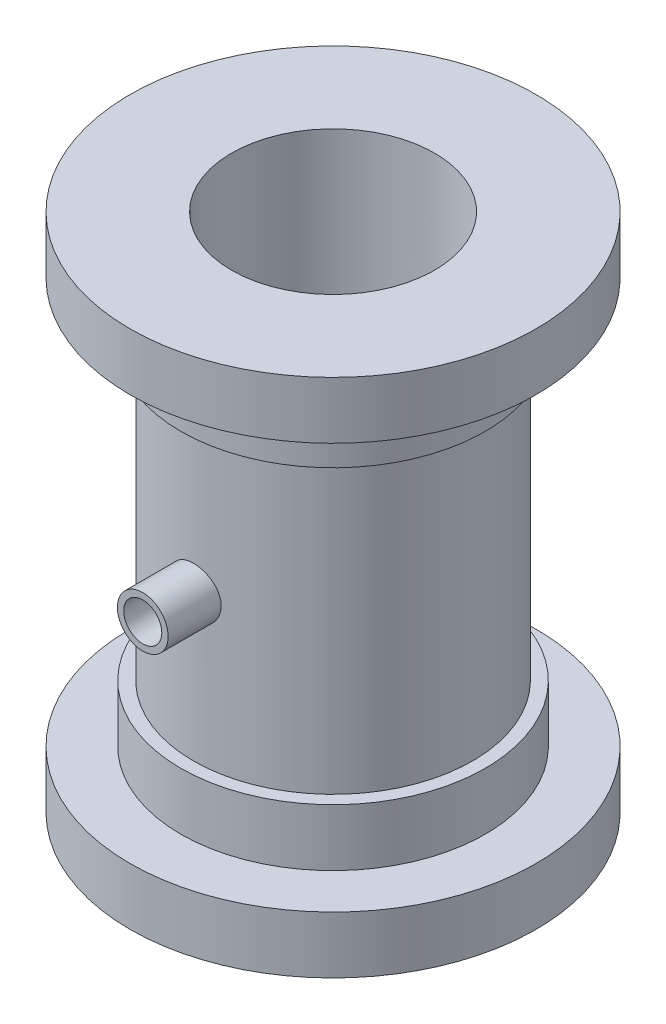
SolidWorks part; units mm, degrees
material "Plain Carbon Steel"
ref_plane "Front Plane" through (0, 0, 0) normal (0, 0, 1) x (1, 0, 0)
ref_plane "Top Plane" through (0, 0, 0) normal (0, 1, 0) x (1, 0, 0)
ref_plane "Right Plane" through (0, 0, 0) normal (1, 0, 0) x (0, 0, -1)
sketch "Spool Profile Sketch" plane through (0, 0, 0) normal (0, 0, 1) x (1, 0, 0)
  line L0 (0, 206.8298) -> (0, -203.2012) construction
  line L1 (16, 82) -> (16, 0)
  line L2 (16, 0) -> (32, 0)
  line L3 (32, 0) -> (32, 9)
  line L4 (32, 9) -> (24, 9)
  line L5 (24, 9) -> (24, 18)
  line L6 (24, 18) -> (22, 18)
  line L7 (22, 18) -> (22, 64)
  line L8 (22, 64) -> (24, 64)
  line L9 (24, 64) -> (24, 73)
  line L10 (24, 73) -> (32, 73)
  line L11 (32, 73) -> (32, 82)
  line L12 (32, 82) -> (16, 82)
  point P5 (32, 4.5)
  dimension "D1" = 82
  dimension "D2" = 46
  dimension "D3" = 9
  dimension "D4" = 16
  dimension "D5" = 22
  dimension "D6" = 24
  dimension "D7" = 32
revolve "Spool Body" add sketch "Spool Profile Sketch" angle 360 about L0
sketch "Side Boss Sketch Ø8" plane through (0, 0, 0) normal (0, 0, 1) x (1, 0, 0)
  circle A0 centre (0, 41) radius 4
  dimension "D1" = 8
  dimension "D2" = 41
extrude "Side Boss Ø8" add sketch "Side Boss Sketch Ø8" along normal blind 30
hole_wizard "Side Boss Cross Hole Ø6" positions "Sketch3" profile "Sketch4" hole size "Ø1.0" standard "ANSI Metric" end condition through all
sketch "Sketch3" plane through (0, 0, 30) normal (0, 0, 1) x (1, 0, 0)
  point P0 (0, 41)
sketch "Sketch4" plane through (0, 41, 30) normal (1, 0, 0) x (0, -1, 0)
  line L0 (0, 0) -> (0, 62)
  line L1 (0, 62) -> (3, 62)
  line L2 (3, 62) -> (3, 0)
  line L5 (3, 0) -> (0, 0)
  line L11 (0, -6.35) -> (0, 107.95) construction
  dimension "Thru Hole Dia." = 6
  dimension "Thru Hole Depth" = 62
hole_wizard "Centre Bore Ø32" positions "Sketch5" profile "Sketch6" hole size "Ø1.0" standard "ANSI Metric" end condition through all
sketch "Sketch5" plane through (0, 82, 0) normal (0, 1, 0) x (1, 0, 0)
  point P0 (0, 0)
sketch "Sketch6" plane through (0, 82, 0) normal (1, 0, 0) x (0, 0, 1)
  line L0 (0, 0) -> (0, 82)
  line L1 (0, 82) -> (16, 82)
  line L2 (16, 82) -> (16, 0)
  line L5 (16, 0) -> (0, 0)
  line L11 (0, -6.35) -> (0, 107.95) construction
  dimension "Thru Hole Dia." = 32
  dimension "Thru Hole Depth" = 82
